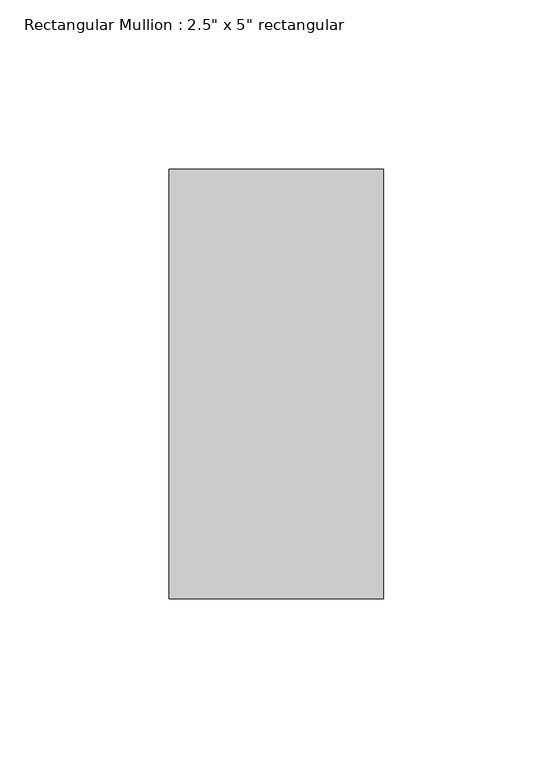
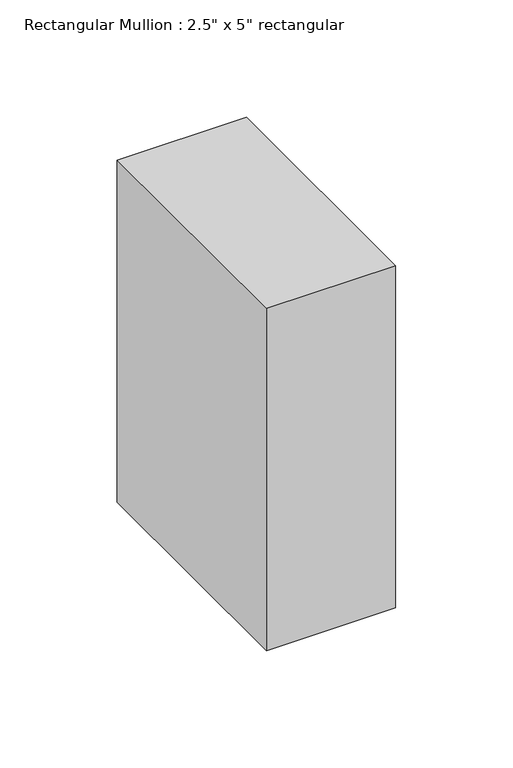
"""IFC4 building model written with IfcOpenShell, lengths in millimetres: member geometry."""

from ifc_helpers import new_model, si_unit, frame, origin, place, context, project, spatial, polyline, outline, extrude, source, transform, mapped, element, save


def member_d92184fb(model_context):
    return source(origin(), model_context, "Body", "SweptSolid", [
        extrude(outline(polyline([(0.0, 63.5), (0.0, -63.5), (-63.5, -63.5), (-63.5, 63.5), (0.0, 63.5)])), frame((0.0, 0.0, -177.8), z_axis=(0.0, 0.0, 1.0), x_axis=(1.0, 0.0, 0.0)), (0.0, 0.0, 1.0), 177.8),
    ])


if __name__ == "__main__":
    model = new_model("IFC4")
    model_context = context("Model", 3, world=origin())
    ifc_project = project(units=[si_unit("LENGTHUNIT", "METRE", prefix="MILLI")], contexts=[model_context])
    site = spatial("IfcSite", under=ifc_project)
    building = spatial("IfcBuilding", under=site)
    placement = place(None, origin())
    member_shape = member_d92184fb(model_context)
    element("IfcMember", 1, ObjectType="Rectangular Mullion : 2.5\" x 5\" rectangular", at=placement, inside=building, context=model_context, shape_type="MappedRepresentation", body=[
        mapped(member_shape, transform((0.0, 0.0, 0.0), x_axis=(1.0, 0.0, 0.0), y_axis=(0.0, 1.0, 0.0), z_axis=(0.0, 0.0, 1.0))),
    ])
    save(model, "model.ifc")

# Revit data of these elements
# Type "Rectangular Mullion : 2.5\" x 5\" rectangular"
#   built-in parameter 1007304 = 0.416667 (stored number, unit not read)
#   built-in parameter 1007301 = 0.104167 (stored number, unit not read)
#   built-in parameter 1007300 = 0.104167 (stored number, unit not read)
# Element 1 (IfcMember, "Rectangular Mullion : 2.5\" x 5\" rectangular")
#   Materials on its faces: "Aluminum"
# Materials
#   "Aluminum": class "Metal", colour RGB 247 247 247, transparency 0, Description = "Aluminum 6061", Cost = 0
